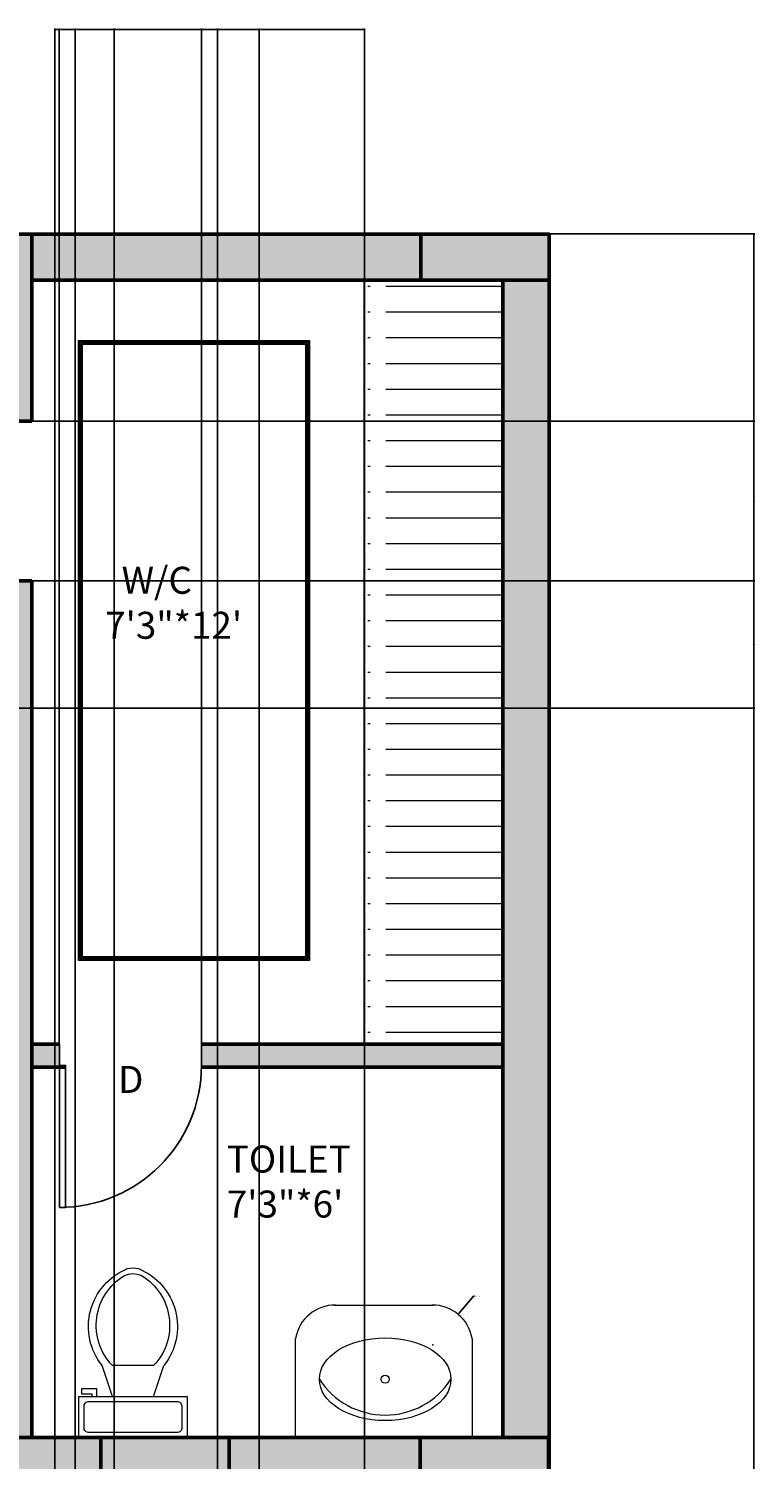
# Model space of a CAD drawing. Units: inches. Extents: x 2494 to 2908, y 1051 to 1885.
# Tile 7 of 7: x 2767 to 2908, y 1607 to 1885. Entities that reach past the tile are written whole.
import ezdxf

# ---------------------------------------------------------------- set-up
doc = ezdxf.new("R2010")
doc.units = ezdxf.units.IN
for name, color, linetype, lineweight in [('A-ANNO-DIMS', 2, 'Continuous', 18), ('A-ANNO-IDEN', 130, 'Continuous', 18), ('A-AREA-IDEN', 130, 'Continuous', 18), ('A-COLS-PATT', 200, 'Continuous', 13), ('A-FLOR-CASE', 230, 'Continuous', 25), ('A-FLOR-FIXT', 230, 'Continuous', 18), ('A-FURN-PATT', 230, 'Continuous', 13), ('A-WALL-PATT', 140, 'Continuous', 13), ('COLUMN', 200, 'Continuous', 50), ('DOOR', 50, 'Continuous', 25), ('FUR', 230, 'Continuous', 18), ('WALL', 140, 'Continuous', 50)]:
    doc.layers.add(name, color=color, linetype=linetype, lineweight=lineweight)
doc.styles.get("Standard").update_dxf_attribs({"font": 'arial.ttf'})
doc.dimstyles.get("Standard").update_dxf_attribs({"dimtxt": 0.18, "dimasz": 0.18, "dimexe": 0.18, "dimexo": 0.0625, "dimgap": 0.09, "dimtad": 0, "dimtih": 1, "dimtoh": 1, "dimdec": 4, "dimzin": 0, "dimdsep": 46, "dimtxsty": 'Standard', "dimcen": 0.09, "dimadec": 0, "dimazin": 0, "dimtfac": 1, "dimtdec": 4, "dimtofl": 0, "dimtmove": 0, "dimatfit": 3, "dimfxl": 1, "dimtolj": 1, "dimtzin": 0, "dimarcsym": 0})

# ---------------------------------------------------------------- blocks, each defined once
blk = doc.blocks.new('*U2')
for p, q in [((0, 0), (0, -6)), ((40, 0), (40, -6))]:
    blk.add_line(p, q)
blk.add_lwpolyline([(0, 0), (0, 40), (1.75, 40), (1.75, 0)], close=True)
blk.add_arc((0, 0), 40, 0, 90)
blk = doc.blocks.new('*U4')
for p, q in [((9.5, -6), (9.5, -2)), ((-8, -8.5), (-8, -8)), ((-7, -8), (-7, -9.5)), ((-4, -8), (-6, -14)), ((4, -8), (6, -14)), ((-10, -8.5), (-8, -8.5)), ((-10, -9.5), (-10, -8.5)), ((-7, -9.5), (-10, -9.5)), ((4, -14), (-4, -14))]:
    blk.add_line(p, q)
blk.add_lwpolyline([(10.5, -8), (10.5, 0), (-10.5, 0), (-10.5, -8)], close=True)
for points in [[(-9.5, -2), (-9.5, -6)], [(8.5, -1), (-8.5, -1)], [(-8.5, -7), (8.5, -7)]]:
    blk.add_lwpolyline(points)
for centre, radius, start, end in [((-8.62, -1.88), 0.884, 81.8699, 188.1301), ((8.62, -1.88), 0.884, 351.8699, 98.1301), ((-8.62, -6.12), 0.884, 171.8699, 278.1301), ((8.62, -6.12), 0.884, 261.8699, 8.1301), ((3.52, -21.58), 12.17, 141.4691, 247.9714), ((4.2, -21.82), 11.33, 136.3677, 238.9468), ((-3.52, -21.58), 12.17, 292.0284, 38.5307), ((-4.2, -21.82), 11.33, 301.053, 43.6321), ((0, -27.88), 4, 245.7318, 294.2682), ((0, -29), 4, 254.8605, 285.1395)]:
    blk.add_arc(centre, radius, start, end)
blk = doc.blocks.new('*D26')
at = {"layer": 'A-ANNO-DIMS', "color": 0, "lineweight": -2, "transparency": 16777216}
for p, q in [((2868.31, 1845.16), (2908.18, 1845.16)), ((2908, 1844.98), (2908, 1468.43)), ((2908, 1091.52), (2908, 1468.07)), ((2860.37, 1091.34), (2908.18, 1091.34))]:
    blk.add_line(p, q, dxfattribs=at)
at = {"layer": 'A-ANNO-DIMS', "color": 0, "lineweight": 100, "transparency": 16777216}
for points in [[(2907.97, 1844.98), (2908.03, 1844.98), (2908, 1845.16)], [(2907.97, 1091.52), (2908.03, 1091.52), (2908, 1091.34)]]:
    blk.add_solid(points, dxfattribs=at)
at = {"layer": 'Defpoints', "color": 0, "lineweight": 100, "transparency": 16777216}
for p in [(2868.25, 1845.16), (2908, 1845.16), (2860.3, 1091.34)]:
    blk.add_point(p, dxfattribs=at)
at = {"layer": 'A-ANNO-DIMS', "color": 0, "transparency": 16777216, "insert": (2908, 1468.25), "char_height": 0.18, "attachment_point": 5}
blk.add_mtext('\\A1;753.8', dxfattribs=at)
blk = doc.blocks.new('*D37')
at = {"layer": 'A-ANNO-DIMS', "color": 0, "lineweight": -2, "transparency": 16777216}
for p, q in [((2783.78, 1155.22), (2783.78, 1885.09)), ((2783.96, 1884.91), (2797.38, 1884.91)), ((2811.73, 1884.91), (2798.31, 1884.91)), ((2811.91, 1155.22), (2811.91, 1885.09))]:
    blk.add_line(p, q, dxfattribs=at)
at = {"layer": 'A-ANNO-DIMS', "color": 0, "lineweight": 100, "transparency": 16777216}
for points in [[(2783.96, 1884.94), (2783.96, 1884.88), (2783.78, 1884.91)], [(2811.73, 1884.94), (2811.73, 1884.88), (2811.91, 1884.91)]]:
    blk.add_solid(points, dxfattribs=at)
at = {"layer": 'Defpoints', "color": 0, "lineweight": 100, "transparency": 16777216}
for p in [(2811.91, 1884.91), (2783.78, 1155.16), (2811.91, 1155.16)]:
    blk.add_point(p, dxfattribs=at)
at = {"layer": 'A-ANNO-DIMS', "color": 0, "transparency": 16777216, "insert": (2797.85, 1884.91), "char_height": 0.18, "attachment_point": 5}
blk.add_mtext('\\A1;28.126', dxfattribs=at)
blk = doc.blocks.new('*D38')
at = {"layer": 'A-ANNO-DIMS', "color": 0, "lineweight": -2, "transparency": 16777216}
for p, q in [((2773.1, 1687.72), (2773.1, 1885.09)), ((2773.28, 1884.91), (2786.44, 1884.91)), ((2800.53, 1884.91), (2787.37, 1884.91)), ((2800.71, 1687.72), (2800.71, 1885.09))]:
    blk.add_line(p, q, dxfattribs=at)
at = {"layer": 'A-ANNO-DIMS', "color": 0, "lineweight": 100, "transparency": 16777216}
for points in [[(2773.28, 1884.94), (2773.28, 1884.88), (2773.1, 1884.91)], [(2800.53, 1884.94), (2800.53, 1884.88), (2800.71, 1884.91)]]:
    blk.add_solid(points, dxfattribs=at)
at = {"layer": 'Defpoints', "color": 0, "lineweight": 100, "transparency": 16777216}
for p in [(2800.71, 1884.91), (2773.1, 1687.66), (2800.71, 1687.66)]:
    blk.add_point(p, dxfattribs=at)
at = {"layer": 'A-ANNO-DIMS', "color": 0, "transparency": 16777216, "insert": (2786.9, 1884.91), "char_height": 0.18, "attachment_point": 5}
blk.add_mtext('\\A1;27.604', dxfattribs=at)
blk = doc.blocks.new('*D43')
at = {"layer": 'A-ANNO-DIMS', "color": 0, "lineweight": -2, "transparency": 16777216}
for p, q in [((2776.2, 1243.72), (2776.2, 1885.09)), ((2776.38, 1884.91), (2789.53, 1884.91)), ((2803.62, 1884.91), (2790.46, 1884.91)), ((2803.8, 1243.72), (2803.8, 1885.09))]:
    blk.add_line(p, q, dxfattribs=at)
at = {"layer": 'A-ANNO-DIMS', "color": 0, "lineweight": 100, "transparency": 16777216}
for points in [[(2776.38, 1884.94), (2776.38, 1884.88), (2776.2, 1884.91)], [(2803.62, 1884.94), (2803.62, 1884.88), (2803.8, 1884.91)]]:
    blk.add_solid(points, dxfattribs=at)
at = {"layer": 'Defpoints', "color": 0, "lineweight": 100, "transparency": 16777216}
for p in [(2803.8, 1884.91), (2776.2, 1243.66), (2803.8, 1243.66)]:
    blk.add_point(p, dxfattribs=at)
at = {"layer": 'A-ANNO-DIMS', "color": 0, "transparency": 16777216, "insert": (2790, 1884.91), "char_height": 0.18, "attachment_point": 5}
blk.add_mtext('\\A1;27.604', dxfattribs=at)
blk = doc.blocks.new('*D44')
at = {"layer": 'A-ANNO-DIMS', "color": 0, "lineweight": -2, "transparency": 16777216}
for p, q in [((2772.25, 1347.22), (2772.25, 1885.09)), ((2772.43, 1884.91), (2801.99, 1884.91)), ((2832.17, 1884.91), (2802.61, 1884.91)), ((2832.35, 1347.22), (2832.35, 1885.09))]:
    blk.add_line(p, q, dxfattribs=at)
at = {"layer": 'A-ANNO-DIMS', "color": 0, "lineweight": 100, "transparency": 16777216}
for points in [[(2772.43, 1884.94), (2772.43, 1884.88), (2772.25, 1884.91)], [(2832.17, 1884.94), (2832.17, 1884.88), (2832.35, 1884.91)]]:
    blk.add_solid(points, dxfattribs=at)
at = {"layer": 'Defpoints', "color": 0, "lineweight": 100, "transparency": 16777216}
for p in [(2832.35, 1884.91), (2772.25, 1347.16), (2832.35, 1347.16)]:
    blk.add_point(p, dxfattribs=at)
at = {"layer": 'A-ANNO-DIMS', "color": 0, "transparency": 16777216, "insert": (2802.3, 1884.91), "char_height": 0.18, "attachment_point": 5}
blk.add_mtext('\\A1;60.1', dxfattribs=at)
blk = doc.blocks.new('*D45')
at = {"layer": 'A-ANNO-DIMS', "color": 0, "lineweight": -2, "transparency": 16777216}
for p, q in [((2767.81, 1808.76), (2908.18, 1808.76)), ((2908, 1808.58), (2908, 1793.43)), ((2908, 1777.91), (2908, 1793.06)), ((2767.81, 1777.73), (2908.18, 1777.73))]:
    blk.add_line(p, q, dxfattribs=at)
at = {"layer": 'A-ANNO-DIMS', "color": 0, "lineweight": 100, "transparency": 16777216}
for points in [[(2907.97, 1808.58), (2908.03, 1808.58), (2908, 1808.76)], [(2907.97, 1777.91), (2908.03, 1777.91), (2908, 1777.73)]]:
    blk.add_solid(points, dxfattribs=at)
at = {"layer": 'Defpoints', "color": 0, "lineweight": 100, "transparency": 16777216}
for p in [(2767.75, 1808.76), (2908, 1808.76), (2767.75, 1777.73)]:
    blk.add_point(p, dxfattribs=at)
at = {"layer": 'A-ANNO-DIMS', "color": 0, "transparency": 16777216, "insert": (2908, 1793.25), "char_height": 0.18, "attachment_point": 5}
blk.add_mtext('\\A1;31.03', dxfattribs=at)
blk = doc.blocks.new('*D67')
at = {"layer": 'A-ANNO-DIMS', "color": 0, "lineweight": -2, "transparency": 16777216}
for p, q in [((2767.81, 1777.73), (2908.18, 1777.73)), ((2908, 1777.55), (2908, 1765.52)), ((2908, 1753.14), (2908, 1765.16)), ((2752.71, 1752.96), (2908.18, 1752.96))]:
    blk.add_line(p, q, dxfattribs=at)
at = {"layer": 'A-ANNO-DIMS', "color": 0, "lineweight": 100, "transparency": 16777216}
for points in [[(2907.97, 1777.55), (2908.03, 1777.55), (2908, 1777.73)], [(2907.97, 1753.14), (2908.03, 1753.14), (2908, 1752.96)]]:
    blk.add_solid(points, dxfattribs=at)
at = {"layer": 'Defpoints', "color": 0, "lineweight": 100, "transparency": 16777216}
for p in [(2767.75, 1777.73), (2908, 1777.73), (2752.64, 1752.96)]:
    blk.add_point(p, dxfattribs=at)
at = {"layer": 'A-ANNO-DIMS', "color": 0, "transparency": 16777216, "insert": (2908, 1765.34), "char_height": 0.18, "attachment_point": 5}
blk.add_mtext('\\A1;24.77', dxfattribs=at)
blk = doc.blocks.new('*D70')
at = {"layer": 'A-ANNO-DIMS', "color": 0, "lineweight": -2, "transparency": 16777216}
for p, q in [((2853.58, 1638.68), (2850.72, 1635.26)), ((2853.76, 1638.68), (2853.58, 1638.68)), ((2845.56, 1629.2), (2845.74, 1629.2)), ((2845.65, 1629.11), (2845.65, 1629.29))]:
    blk.add_line(p, q, dxfattribs=at)
at = {"layer": 'A-ANNO-DIMS', "color": 0, "lineweight": 100, "transparency": 16777216}
blk.add_solid([(2850.7, 1635.28), (2850.75, 1635.24), (2850.61, 1635.12)], dxfattribs=at)
at = {"layer": 'Defpoints', "color": 0, "lineweight": 100, "transparency": 16777216}
for p in [(2850.61, 1635.12), (2845.65, 1629.2)]:
    blk.add_point(p, dxfattribs=at)
at = {"layer": 'A-ANNO-DIMS', "color": 0, "transparency": 16777216, "insert": (2854.37, 1638.68), "char_height": 0.18, "attachment_point": 5}
blk.add_mtext('\\A1;4X R7.72', dxfattribs=at)

msp = doc.modelspace()

# ---------------------------------------------------------------- hatches: boundary and pattern name
at = {"layer": 'A-COLS-PATT'}
h = msp.add_hatch(color=256, dxfattribs=at)
h.dxf.hatch_style = 1
h.paths.add_polyline_path([(2584.1612, 1845.1561), (2559.2517, 1845.1561), (2559.2517, 1836.1561), (2584.1612, 1836.1561)])
h.paths.add_polyline_path([(2720.7462, 1845.1561), (2695.8368, 1845.1561), (2695.8368, 1836.1561), (2720.7462, 1836.1561)])
h.paths.add_polyline_path([(2868.2517, 1845.1561), (2843.3423, 1845.1561), (2843.3423, 1836.1561), (2868.2517, 1836.1561)])
h.paths.add_polyline_path([(2568.2517, 1728.1561), (2559.2517, 1728.1561), (2559.2517, 1703.2467), (2568.2517, 1703.2467)])
h.paths.add_polyline_path([(2568.2517, 1564.0885), (2559.2517, 1564.0885), (2559.2517, 1539.1791), (2568.2517, 1539.1791)])
h.paths.add_polyline_path([(2868.2517, 1554.4528), (2859.2517, 1554.4528), (2859.2517, 1529.5434), (2868.2517, 1529.5434)])
h.paths.add_polyline_path([(2806.0841, 1611.1561), (2781.1746, 1611.1561), (2781.1746, 1602.1561), (2806.0841, 1602.1561)])
h.paths.add_polyline_path([(2868.0971, 1611.1561), (2843.1877, 1611.1561), (2843.1877, 1602.1561), (2868.0971, 1602.1561)])
h.paths.add_polyline_path([(2584.1612, 1347.1561), (2559.2517, 1347.1561), (2559.2517, 1338.1561), (2584.1612, 1338.1561)])
h.paths.add_polyline_path([(2868.2517, 1347.1561), (2843.3423, 1347.1561), (2843.3423, 1338.1561), (2868.2517, 1338.1561)])
h.paths.add_polyline_path([(2568.2517, 1180.0656), (2559.2517, 1180.0656), (2559.2517, 1155.1561), (2568.2517, 1155.1561)])
h.paths.add_polyline_path([(2584.1612, 1155.1561), (2559.2517, 1155.1561), (2559.2517, 1146.1561), (2584.1612, 1146.1561)])
h.paths.add_polyline_path([(2868.2517, 1155.1561), (2843.3423, 1155.1561), (2843.3423, 1146.1561), (2868.2517, 1146.1561)])
h.paths.add_polyline_path([(2868.2517, 1180.0656), (2859.2517, 1180.0656), (2859.2517, 1155.1561), (2868.2517, 1155.1561)])
at = {"layer": 'A-FURN-PATT'}
h = msp.add_hatch(dxfattribs=at)
h.set_pattern_fill('ACAD_ISO04W100', color=256)
h.paths.add_polyline_path([(2763.2517, 1836.1561), (2568.2517, 1836.1561), (2568.2517, 1811.916), (2763.2517, 1811.916)])
h.paths.add_polyline_path([(2859.2517, 1836.1561), (2843.3423, 1836.1561), (2832.2996, 1836.1561), (2832.2996, 1687.6561), (2859.2517, 1687.6561)])
h.paths.add_polyline_path([(2859.2517, 1338.1485), (2840.7638, 1338.1485), (2840.7638, 1243.6561), (2859.2517, 1243.6561)])
at = {"layer": 'A-WALL-PATT'}
h = msp.add_hatch(color=256, dxfattribs=at)
h.dxf.hatch_style = 1
h.paths.add_polyline_path([(2609.6092, 1845.1561), (2584.1612, 1845.1561), (2584.1612, 1836.1561), (2609.6092, 1836.1561)])
h.paths.add_polyline_path([(2695.8368, 1845.1561), (2672.7564, 1845.1561), (2672.7564, 1836.1561), (2695.8368, 1836.1561)])
h.paths.add_polyline_path([(2767.7517, 1845.1561), (2720.7462, 1845.1561), (2720.7462, 1836.1561), (2763.2517, 1836.1561), (2763.2517, 1808.7615), (2767.7517, 1808.7615)])
h.paths.add_polyline_path([(2843.3423, 1845.1561), (2767.7517, 1845.1561), (2767.7517, 1836.1561), (2843.3423, 1836.1561)])
h.paths.add_polyline_path([(2568.2517, 1836.1561), (2559.2517, 1836.1561), (2559.2517, 1728.1561), (2568.2517, 1728.1561)])
h.paths.add_polyline_path([(2568.2517, 1703.2467), (2559.2517, 1703.2467), (2559.2517, 1611.1561), (2568.2517, 1611.1561)])
h.paths.add_polyline_path([(2843.1877, 1611.1561), (2819.0012, 1611.1561), (2806.0841, 1611.1561), (2806.0841, 1602.1561), (2843.1877, 1602.1561)])
h.paths.add_polyline_path([(2805.2517, 1602.1561), (2796.2517, 1602.1561), (2796.2517, 1591.2367), (2805.2517, 1591.2367)])
h = msp.add_hatch(color=256, dxfattribs=at)
h.dxf.hatch_style = 1
h.paths.add_polyline_path([(2868.2517, 1836.1561), (2859.2517, 1836.1561), (2859.2517, 1611.1561), (2868.2517, 1611.1561)])
h.paths.add_polyline_path([(2715.2517, 1611.1561), (2655.4916, 1611.1561), (2655.4916, 1606.6561), (2715.2517, 1606.6561)])
h.paths.add_polyline_path([(2781.1746, 1611.1561), (2776.9029, 1611.1561), (2715.2517, 1611.1561), (2715.2517, 1606.6561), (2715.2517, 1602.1561), (2781.1746, 1602.1561)])
h.paths.add_polyline_path([(2868.0971, 1602.1561), (2859.2517, 1602.1561), (2859.2517, 1554.4528), (2868.0971, 1554.4528)])
h.paths.add_polyline_path([(2868.2517, 1529.5434), (2859.2517, 1529.5434), (2859.2517, 1347.1561), (2868.2517, 1347.1561)])
h.paths.add_polyline_path([(2868.2517, 1338.1561), (2859.2517, 1338.1561), (2859.2517, 1243.6561), (2868.2517, 1243.6561)])
h.paths.add_polyline_path([(2568.2517, 1338.1561), (2559.2517, 1338.1561), (2559.2517, 1180.0656), (2568.2517, 1180.0656)])
h.paths.add_polyline_path([(2735.7191, 1155.1561), (2697.838, 1155.1561), (2697.838, 1146.1561), (2735.7191, 1146.1561), (2735.7191, 1151.0155)])
h = msp.add_hatch(color=256, dxfattribs=at)
h.dxf.hatch_style = 1
h.paths.add_polyline_path([(2767.7517, 1777.7287), (2763.2517, 1777.7287), (2763.2517, 1611.1561), (2767.7517, 1611.1561), (2767.7517, 1683.1561)])
h = msp.add_hatch(color=256, dxfattribs=at)
h.dxf.hatch_style = 1
h.paths.add_polyline_path([(2859.2517, 1687.6561), (2800.7065, 1687.6561), (2800.7065, 1683.5155, -0.00325461), (2800.7041, 1683.1561), (2859.2517, 1683.1561)])
h.paths.add_polyline_path([(2773.1022, 1687.6561), (2767.7517, 1687.6561), (2767.7517, 1683.1561), (2773.1022, 1683.1561), (2773.1022, 1683.5155)])

# ---------------------------------------------------------------- linework, layer by layer
at = {"layer": 'A-FLOR-CASE'}
msp.add_line((2832.2996, 1687.6561), (2832.2996, 1836.1561), dxfattribs=at)
at = {"layer": 'A-FLOR-FIXT'}
for points in [[(2826.5093, 1636.9217), (2845.7646, 1636.9217)], [(2853.2727, 1630.4567), (2853.2727, 1611.1561), (2819.0012, 1611.1561), (2819.0012, 1630.4567)]]:
    msp.add_lwpolyline(points, dxfattribs=at)
msp.add_circle((2836.3955, 1622.5091), 0.7921, dxfattribs=at)
for centre, radius, start, end in [((2826.6193, 1629.2017), 7.7207, 89.183797, 170.645503), ((2845.6546, 1629.2017), 7.7207, 9.354497, 90.816203), ((2836.3955, 1630.753), 15.2147, 212.808997, 327.191003)]:
    msp.add_arc(centre, radius, start, end, dxfattribs=at)
msp.add_ellipse((2836.3955, 1622.5091), major_axis=(12.7877, 0), ratio=0.62936955, dxfattribs=at)
at = {"layer": 'COLUMN'}
for points in [[(2843.3423, 1845.1561), (2868.2517, 1845.1561), (2868.2517, 1836.1561), (2843.3423, 1836.1561)], [(2781.1746, 1611.1561), (2806.0841, 1611.1561), (2806.0841, 1602.1561), (2781.1746, 1602.1561)], [(2843.1877, 1611.1561), (2868.0971, 1611.1561), (2868.0971, 1602.1561), (2843.1877, 1602.1561)]]:
    msp.add_lwpolyline(points, close=True, dxfattribs=at)
at = {"layer": 'FUR'}
for points in [[(2776.8478, 1824.4777), (2821.6729, 1824.4777), (2821.6729, 1703.8945), (2776.8478, 1703.8945)], [(2777.0978, 1824.2277), (2821.4229, 1824.2277), (2821.4229, 1704.1445), (2777.0978, 1704.1445)], [(2777.3478, 1823.9777), (2821.1729, 1823.9777), (2821.1729, 1704.3945), (2777.3478, 1704.3945)], [(2777.5978, 1823.7277), (2820.9229, 1823.7277), (2820.9229, 1704.6445), (2777.5978, 1704.6445)]]:
    msp.add_lwpolyline(points, close=True, dxfattribs=at)
at = {"layer": 'WALL'}
for p, q in [((2559.2517, 1845.1561), (2767.7517, 1845.1561)), ((2767.7517, 1845.1561), (2767.7517, 1808.7615)), ((2868.2517, 1845.1561), (2767.7517, 1845.1561)), ((2868.2517, 1611.1561), (2868.2517, 1845.1561)), ((2859.2517, 1836.1561), (2767.7517, 1836.1561)), ((2859.2517, 1611.1561), (2859.2517, 1836.1561)), ((2767.7517, 1777.7287), (2767.7517, 1611.1561)), ((2767.7517, 1687.6561), (2773.1022, 1687.6561)), ((2800.7065, 1687.6561), (2859.2517, 1687.6561)), ((2767.7517, 1611.1561), (2767.7517, 1683.1561)), ((2767.7517, 1683.1561), (2774.3098, 1683.1561)), ((2800.7041, 1683.1561), (2859.2517, 1683.1561)), ((2854.7517, 1683.1561), (2859.2517, 1683.1561)), ((2868.2517, 1611.1561), (2719.7517, 1611.1561)), ((2868.2517, 1347.1561), (2868.2517, 1611.1561))]:
    msp.add_line(p, q, dxfattribs=at)
for points in [[(2859.2517, 1611.1561), (2868.2517, 1611.1561), (2868.2517, 1836.1561), (2859.2517, 1836.1561)], [(2715.2517, 1602.1561), (2781.1746, 1602.1561), (2781.1746, 1611.1561), (2715.2517, 1611.1561)]]:
    msp.add_lwpolyline(points, close=True, dxfattribs=at)
for points in [[(2763.2517, 1808.7615), (2767.7517, 1808.7615)], [(2767.7517, 1777.7287), (2763.2517, 1777.7287)]]:
    msp.add_lwpolyline(points, dxfattribs=at)

# ---------------------------------------------------------------- block references
at = {"layer": 'A-FLOR-FIXT', "xscale": -1, "rotation": 180}
msp.add_blockref('*U4', (2787.4029, 1611.1561), dxfattribs=at)
at = {"layer": 'DOOR', "xscale": -0.6901078009918955, "yscale": 0.6901078009918955, "zscale": 0.6901078009918955, "rotation": 180}
msp.add_blockref('*U2', (2773.1022, 1683.5155), dxfattribs=at)

# ---------------------------------------------------------------- texts
at = {"layer": 'A-ANNO-IDEN', "insert": (2784.5123, 1683.4105), "char_height": 5.2482, "attachment_point": 1}
msp.add_mtext_dynamic_manual_height_columns('D', width=250.978097, gutter_width=26.2409, heights=[0], dxfattribs=at)
at = {"layer": 'A-AREA-IDEN', "char_height": 5.24818, "attachment_point": 1}
for s, insert in [('  W/C\\P7\'3"*12\'', (2781.9968, 1780.4594)), ('TOILET\\P7\'3"*6\'', (2805.6291, 1667.9345))]:
    msp.add_mtext_dynamic_manual_height_columns(s, width=250.978097, gutter_width=26.2409, heights=[0], dxfattribs=dict(at, insert=insert))

# ---------------------------------------------------------------- dimensions: what is measured, and where the dimension line sits
at = {"layer": 'A-ANNO-DIMS'}
for base, p1, p2, override, picture, middle in [((2832.3482, 1884.9061), (2772.2517, 1347.1561), (2832.3482, 1347.1561), {"dimdec": 1, "dimlfac": 1, "dimrnd": 0, "dimzin": 0, "dimdsep": 46, "dimlunit": 2}, '*D44', (2802.3, 1884.9061)), ((2800.7065, 1884.9061), (2773.1022, 1687.6561), (2800.7065, 1687.6561), {"dimdec": 3, "dimlfac": 1, "dimrnd": 0, "dimzin": 0, "dimdsep": 46, "dimlunit": 2}, '*D38', (2786.9043, 1884.9061)), ((2803.8003, 1884.9061), (2776.196, 1243.6561), (2803.8003, 1243.6561), {"dimdec": 3, "dimlfac": 1, "dimrnd": 0, "dimzin": 0, "dimdsep": 46, "dimlunit": 2}, '*D43', (2789.9982, 1884.9061)), ((2811.9091, 1884.9061), (2783.7833, 1155.1561), (2811.9091, 1155.1561), {"dimdec": 3, "dimlfac": 1, "dimrnd": 0, "dimzin": 0, "dimdsep": 46, "dimlunit": 2}, '*D37', (2797.8462, 1884.9061))]:
    dim = msp.add_linear_dim(base=base, p1=p1, p2=p2, dimstyle='Standard', override=override, dxfattribs=at)
    dim.commit()
    dim.dimension.update_dxf_attribs({"geometry": picture, "text_midpoint": middle})
for base, p1, p2, override, picture, middle in [((2908.0017, 1845.1561), (2860.3038, 1091.3437), (2868.2517, 1845.1561), {"dimdec": 1, "dimlfac": 1, "dimrnd": 0, "dimzin": 0, "dimdsep": 46, "dimlunit": 2}, '*D26', (2908.0017, 1468.2499)), ((2908.0017, 1808.7615), (2767.7517, 1777.7287), (2767.7517, 1808.7615), {"dimdec": 2, "dimlfac": 1, "dimrnd": 0, "dimzin": 0, "dimdsep": 46, "dimlunit": 2}, '*D45', (2908.0017, 1793.2451)), ((2908.0017, 1777.7287), (2752.6447, 1752.9565), (2767.7517, 1777.7287), {"dimdec": 2, "dimlfac": 1, "dimrnd": 0, "dimzin": 0, "dimdsep": 46, "dimlunit": 2}, '*D67', (2908.0017, 1765.3426))]:
    dim = msp.add_linear_dim(base=base, p1=p1, p2=p2, angle=90, dimstyle='Standard', override=override, dxfattribs=at)
    dim.commit()
    dim.dimension.update_dxf_attribs({"geometry": picture, "text_midpoint": middle})
dim = msp.add_radius_dim(center=(2845.6546, 1629.2017), mpoint=(2850.6086, 1635.1235), text='4X <>', dimstyle='Standard', override={"dimdec": 2, "dimlfac": 1, "dimrnd": 0, "dimzin": 0, "dimdsep": 46, "dimlunit": 2}, dxfattribs=at)
dim.commit()
dim.dimension.update_dxf_attribs({"geometry": '*D70', "text_midpoint": (2854.367, 1638.6766), "dimtype": 164})

doc.saveas('drawing.dxf')
